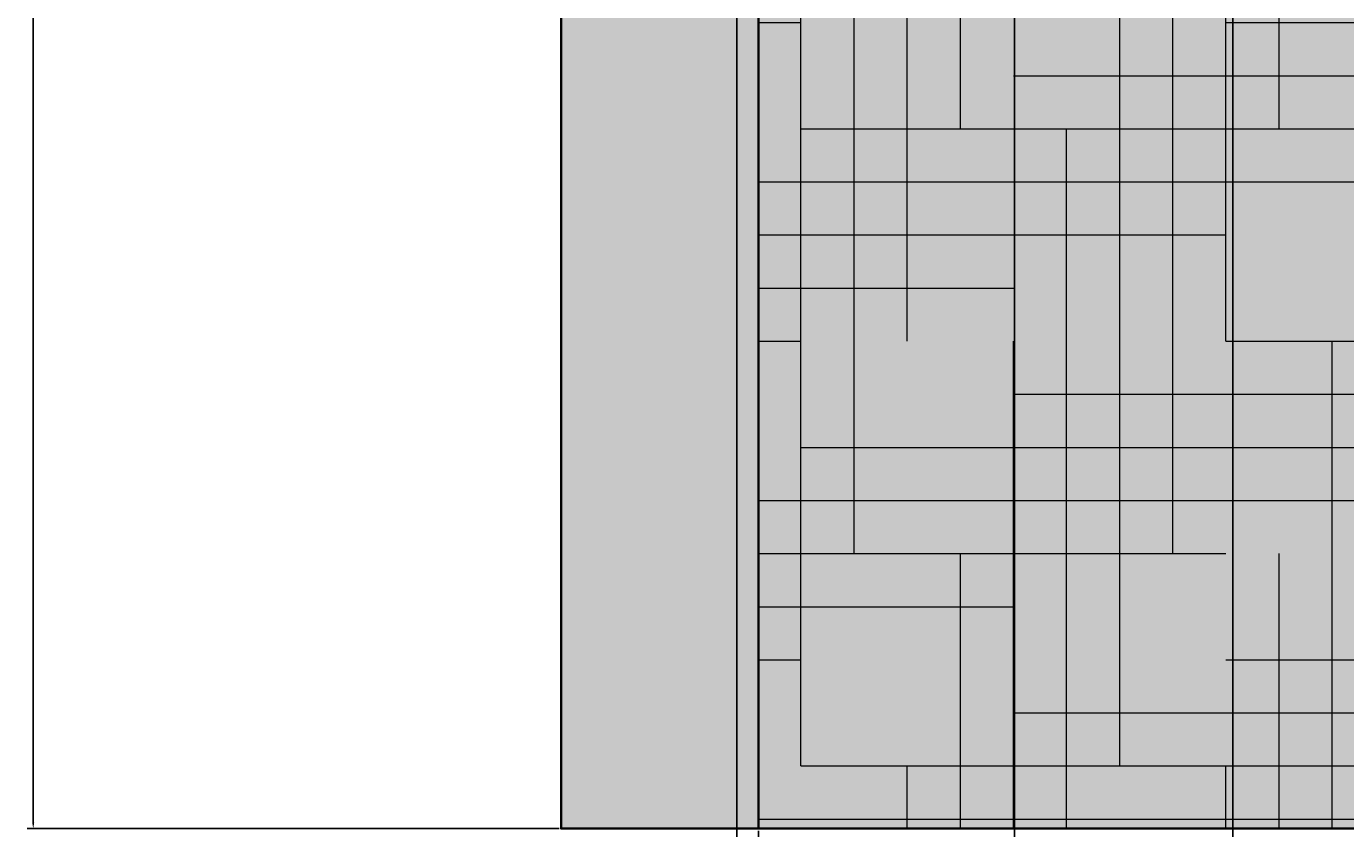
# Model space of a CAD drawing. Units: feet. Extents: x 2695 to 2912, y 795 to 1139.
# Tile 2 of 83: x 2695 to 2734, y 811 to 835. Entities that reach past the tile are written whole.
import ezdxf

# ---------------------------------------------------------------- set-up
doc = ezdxf.new("R2010")
doc.units = ezdxf.units.FT
for name, color, linetype, lineweight in [('A-ANNO-DIMS', 2, 'Continuous', 18), ('A-ELEV', 7, 'Continuous', 35), ('A-ELEV-PATT', 252, 'Continuous', 13)]:
    doc.layers.add(name, color=color, linetype=linetype, lineweight=lineweight)
doc.styles.get("Standard").update_dxf_attribs({"font": 'arial.ttf'})
doc.dimstyles.get("Standard").update_dxf_attribs({"dimtxt": 0.18, "dimasz": 0.18, "dimexe": 0.18, "dimexo": 0.0625, "dimgap": 0.09, "dimtad": 0, "dimtih": 1, "dimtoh": 1, "dimdec": 1, "dimzin": 0, "dimdsep": 46, "dimlunit": 3, "dimtxsty": 'Standard', "dimcen": 0.09, "dimadec": 0, "dimazin": 0, "dimtfac": 1, "dimtdec": 1, "dimtofl": 0, "dimtmove": 0, "dimatfit": 3, "dimfxl": 1, "dimtolj": 1, "dimtzin": 0, "dimarcsym": 0})

# ---------------------------------------------------------------- blocks, each defined once
blk = doc.blocks.new('*D2')
at = {"layer": 'A-ANNO-DIMS', "color": 0, "lineweight": -2, "transparency": 16777216}
for p, q in [((2724.189, 874.795), (2724.189, 794.976)), ((2716.536, 810.868), (2716.536, 794.976)), ((2716.716, 795.156), (2719.97, 795.156)), ((2724.009, 795.156), (2720.756, 795.156))]:
    blk.add_line(p, q, dxfattribs=at)
at = {"layer": 'A-ANNO-DIMS', "color": 0, "transparency": 16777216}
for points in [[(2716.716, 795.186), (2716.716, 795.126), (2716.536, 795.156)], [(2724.009, 795.186), (2724.009, 795.126), (2724.189, 795.156)]]:
    blk.add_solid(points, dxfattribs=at)
at = {"layer": 'Defpoints', "color": 0, "transparency": 16777216}
for p in [(2724.189, 874.857), (2716.536, 810.931), (2724.189, 795.156)]:
    blk.add_point(p, dxfattribs=at)
at = {"layer": 'A-ANNO-DIMS', "color": 0, "transparency": 16777216, "insert": (2720.363, 795.156), "char_height": 0.18, "attachment_point": 5}
blk.add_mtext('\\A1;7.653', dxfattribs=at)
blk = doc.blocks.new('*D3')
at = {"layer": 'A-ANNO-DIMS', "color": 0, "lineweight": -2, "transparency": 16777216}
for p, q in [((2724.189, 874.795), (2724.189, 794.976)), ((2758.151, 874.795), (2758.151, 794.976)), ((2724.369, 795.156), (2740.777, 795.156)), ((2757.971, 795.156), (2741.564, 795.156))]:
    blk.add_line(p, q, dxfattribs=at)
at = {"layer": 'A-ANNO-DIMS', "color": 0, "transparency": 16777216}
for points in [[(2724.369, 795.186), (2724.369, 795.126), (2724.189, 795.156)], [(2757.971, 795.186), (2757.971, 795.126), (2758.151, 795.156)]]:
    blk.add_solid(points, dxfattribs=at)
at = {"layer": 'Defpoints', "color": 0, "transparency": 16777216}
for p in [(2724.189, 874.857), (2758.151, 874.857), (2758.151, 795.156)]:
    blk.add_point(p, dxfattribs=at)
at = {"layer": 'A-ANNO-DIMS', "color": 0, "transparency": 16777216, "insert": (2741.17, 795.156), "char_height": 0.18, "attachment_point": 5}
blk.add_mtext('\\A1;33.96', dxfattribs=at)
blk = doc.blocks.new('*D12')
at = {"layer": 'A-ANNO-DIMS', "color": 0, "lineweight": -2, "transparency": 16777216}
for p, q in [((2710.574, 1122.931), (2694.681, 1122.931)), ((2694.861, 1122.751), (2694.861, 967.113)), ((2694.861, 811.111), (2694.861, 966.749)), ((2710.574, 810.931), (2694.681, 810.931))]:
    blk.add_line(p, q, dxfattribs=at)
at = {"layer": 'A-ANNO-DIMS', "color": 0, "transparency": 16777216}
for points in [[(2694.831, 1122.751), (2694.891, 1122.751), (2694.861, 1122.931)], [(2694.831, 811.111), (2694.891, 811.111), (2694.861, 810.931)]]:
    blk.add_solid(points, dxfattribs=at)
at = {"layer": 'Defpoints', "color": 0, "transparency": 16777216}
for p in [(2694.861, 1122.931), (2710.636, 1122.931), (2710.636, 810.931)]:
    blk.add_point(p, dxfattribs=at)
at = {"layer": 'A-ANNO-DIMS', "color": 0, "transparency": 16777216, "insert": (2694.861, 966.931), "char_height": 0.18, "attachment_point": 5}
blk.add_mtext('\\A1;312', dxfattribs=at)
blk = doc.blocks.new('*D23')
at = {"layer": 'A-ANNO-DIMS', "color": 0, "lineweight": -2, "transparency": 16777216}
for p, q in [((2715.885, 936.868), (2715.885, 794.976)), ((2730.708, 936.868), (2730.708, 794.976)), ((2716.065, 795.156), (2722.842, 795.156)), ((2730.528, 795.156), (2723.752, 795.156))]:
    blk.add_line(p, q, dxfattribs=at)
at = {"layer": 'A-ANNO-DIMS', "color": 0, "transparency": 16777216}
for points in [[(2716.065, 795.186), (2716.065, 795.126), (2715.885, 795.156)], [(2730.528, 795.186), (2730.528, 795.126), (2730.708, 795.156)]]:
    blk.add_solid(points, dxfattribs=at)
at = {"layer": 'Defpoints', "color": 0, "transparency": 16777216}
for p in [(2715.885, 936.931), (2730.708, 936.931), (2730.708, 795.156)]:
    blk.add_point(p, dxfattribs=at)
at = {"layer": 'A-ANNO-DIMS', "color": 0, "transparency": 16777216, "insert": (2723.297, 795.156), "char_height": 0.18, "attachment_point": 5}
blk.add_mtext('\\A1;14.823', dxfattribs=at)
blk = doc.blocks.new('*D24')
at = {"layer": 'A-ANNO-DIMS', "color": 0, "lineweight": -2, "transparency": 16777216}
for p, q in [((2730.708, 936.868), (2730.708, 794.976)), ((2755.112, 936.868), (2755.112, 794.976)), ((2730.888, 795.156), (2742.446, 795.156)), ((2754.932, 795.156), (2743.375, 795.156))]:
    blk.add_line(p, q, dxfattribs=at)
at = {"layer": 'A-ANNO-DIMS', "color": 0, "transparency": 16777216}
for points in [[(2730.888, 795.186), (2730.888, 795.126), (2730.708, 795.156)], [(2754.932, 795.186), (2754.932, 795.126), (2755.112, 795.156)]]:
    blk.add_solid(points, dxfattribs=at)
at = {"layer": 'Defpoints', "color": 0, "transparency": 16777216}
for p in [(2730.708, 936.931), (2755.112, 936.931), (2755.112, 795.156)]:
    blk.add_point(p, dxfattribs=at)
at = {"layer": 'A-ANNO-DIMS', "color": 0, "transparency": 16777216, "insert": (2742.91, 795.156), "char_height": 0.18, "attachment_point": 5}
blk.add_mtext('\\A1;24.404', dxfattribs=at)

msp = doc.modelspace()

# ---------------------------------------------------------------- hatches: boundary and pattern name
at = {"layer": 'A-ELEV-PATT'}
h = msp.add_hatch(color=256, dxfattribs=at)
h.set_gradient(color1=(255, 255, 255), tint=1)
h.paths.add_polyline_path([(2770.6361, 1122.9306), (2710.6361, 1122.9306), (2710.6361, 1118.4096), (2770.6361, 1118.4096)])
h.paths.add_polyline_path([(2890.6361, 1107.8588), (2770.6361, 1107.8588), (2770.6361, 1103.3378), (2890.6361, 1103.3378)])
h.paths.add_polyline_path([(2890.6361, 1062.9306), (2710.6361, 1062.9306), (2710.6361, 1056.9306), (2710.6361, 936.9306), (2710.6361, 924.3105), (2716.5358, 924.3105), (2890.6361, 924.3105), (2890.6361, 936.9306), (2715.8852, 936.9306), (2715.8852, 1050.3105), (2890.6361, 1050.3105)])
h.paths.add_polyline_path([(2716.5358, 924.3105), (2710.6361, 924.3105), (2710.6361, 810.9306), (2716.5358, 810.9306)])
h = msp.add_hatch(color=256, dxfattribs=at)
h.set_gradient(color1=(255, 255, 255))
h.paths.add_polyline_path([(2770.6361, 924.3105), (2716.5358, 924.3105), (2716.5358, 810.9306), (2770.6361, 810.9306)])
h.paths.add_polyline_path([(2758.1515, 902.577), (2758.1515, 874.8571), (2724.1893, 874.8571), (2724.1893, 902.577)], flags=16)
h.paths.add_polyline_path([(2756.1515, 900.577), (2756.1515, 876.8571), (2726.1893, 876.8571), (2726.1893, 900.577)], flags=0)
h.paths.add_polyline_path([(2740.7302, 900.577), (2741.6105, 900.577), (2741.6105, 876.8571), (2740.7302, 876.8571)], flags=0)
h = msp.add_hatch(dxfattribs=at)
h.set_pattern_fill('HOUND', color=256, style=0)
h.paths.add_polyline_path([(2770.6361, 924.3105), (2716.5358, 924.3105), (2716.5358, 810.9306), (2770.6361, 810.9306)])
h.paths.add_polyline_path([(2724.1893, 874.8571), (2724.1893, 902.577), (2758.1515, 902.577), (2758.1515, 874.8571)], flags=16)
h.paths.add_polyline_path([(2756.1515, 876.8571), (2726.1893, 876.8571), (2726.1893, 900.577), (2756.1515, 900.577)], flags=0)
h.paths.add_polyline_path([(2741.6105, 876.8571), (2740.7302, 876.8571), (2740.7302, 900.577), (2741.6105, 900.577)], flags=0)

# ---------------------------------------------------------------- linework, layer by layer
at = {"layer": 'A-ELEV'}
for p, q in [((2710.6361, 930.9306), (2710.6361, 810.9306)), ((2716.5358, 924.3105), (2716.5358, 810.9306)), ((2710.6361, 810.9306), (2890.6361, 810.9306)), ((2710.6361, 810.9306), (2890.6361, 810.9306)), ((2710.6361, 810.9306), (2895.4426, 810.9306)), ((2716.5358, 810.9306), (2770.6361, 810.9306))]:
    msp.add_line(p, q, dxfattribs=at)
for points in [[(2710.6361, 924.3105), (2716.5358, 924.3105), (2716.5358, 810.9306), (2710.6361, 810.9306)], [(2716.5358, 924.3105), (2770.6361, 924.3105), (2770.6361, 810.9306), (2716.5358, 810.9306)]]:
    msp.add_lwpolyline(points, close=True, dxfattribs=at)

# ---------------------------------------------------------------- dimensions: what is measured, and where the dimension line sits
at = {"layer": 'A-ANNO-DIMS'}
dim = msp.add_linear_dim(base=(2694.8611, 1122.9306), p1=(2710.6361, 810.9306), p2=(2710.6361, 1122.9306), angle=90, dimstyle='Standard', override={"dimdec": 0, "dimlfac": 1, "dimrnd": 0, "dimzin": 0, "dimdsep": 46, "dimlunit": 2}, dxfattribs=at)
dim.commit()
dim.dimension.update_dxf_attribs({"geometry": '*D12', "text_midpoint": (2694.8611, 966.9306)})
for base, p1, p2, override, picture, middle in [((2730.7081, 795.1556), (2715.8852, 936.9306), (2730.7081, 936.9306), {"dimdec": 3, "dimlfac": 1, "dimrnd": 0, "dimzin": 0, "dimdsep": 46, "dimlunit": 2}, '*D23', (2723.2967, 795.1556)), ((2755.1125, 795.1556), (2730.7081, 936.9306), (2755.1125, 936.9306), {"dimdec": 3, "dimlfac": 1, "dimrnd": 0, "dimzin": 0, "dimdsep": 46, "dimlunit": 2}, '*D24', (2742.9103, 795.1556)), ((2724.18927, 795.15559), (2716.53582, 810.93059), (2724.18927, 874.85709), {"dimdec": 3, "dimlfac": 1, "dimrnd": 0, "dimzin": 0, "dimdsep": 46, "dimlunit": 2}, '*D2', (2720.36254, 795.15559)), ((2758.1515, 795.1556), (2724.1893, 874.8571), (2758.1515, 874.8571), {"dimdec": 2, "dimlfac": 1, "dimrnd": 0, "dimzin": 0, "dimdsep": 46, "dimlunit": 2}, '*D3', (2741.1704, 795.1556))]:
    dim = msp.add_linear_dim(base=base, p1=p1, p2=p2, dimstyle='Standard', override=override, dxfattribs=at)
    dim.commit()
    dim.dimension.update_dxf_attribs({"geometry": picture, "text_midpoint": middle})

doc.saveas('drawing.dxf')
